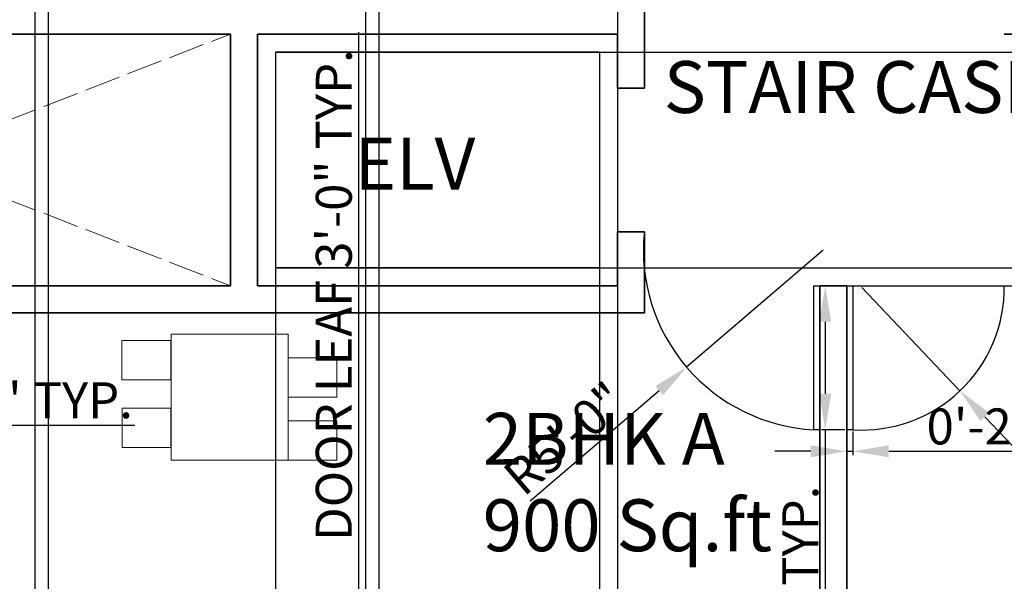
# Model space of a CAD drawing. Units: inches. Extents: x 2174 to 3353, y 1481 to 2316.
# Tile 3 of 8: x 2431 to 2759, y 1713 to 1900. Entities that reach past the tile are written whole.
import ezdxf

# ---------------------------------------------------------------- set-up
doc = ezdxf.new("R2010")
doc.units = ezdxf.units.IN
doc.linetypes.add('ACAD_ISO02W100', pattern=[15, 12, -3])
for name, color, linetype, lineweight in [('A-ANNO-DIMS', 2, 'Continuous', 18), ('A-AREA-IDEN', 7, 'Continuous', 25), ('A-DOOR', 4, 'Continuous', 25), ('A-EQPM-ELEV', 4, 'Continuous', 25), ('A-FLOR-OPEN', 8, 'ACAD_ISO02W100', 13), ('A-FURN', 8, 'Continuous', 13), ('A-WALL', 7, 'Continuous', 35)]:
    doc.layers.add(name, color=color, linetype=linetype, lineweight=lineweight)
doc.styles.get("Standard").update_dxf_attribs({"font": 'arial.ttf'})
doc.dimstyles.new('ISO-25', dxfattribs={"dimtxt": 12, "dimasz": 12, "dimexe": 1.25, "dimexo": 0.625, "dimtad": 1, "dimlunit": 3, "dimtxsty": 'Standard', "dimcen": 2.5, "dimadec": 0, "dimazin": 0, "dimtfac": 1, "dimtmove": 0, "dimatfit": 3, "dimfxl": 1, "dimarcsym": 0})

# ---------------------------------------------------------------- blocks, each defined once
blk = doc.blocks.new('DINING-SET-4')
for points in [[(0, 39.9), (16.26, 39.9), (16.26, 26.81), (0, 26.81)], [(16.43, 42.05), (55.41, 42.05), (55.41, 0), (16.43, 0)], [(55.41, 34.11), (71.67, 34.11), (71.67, 21.03), (55.41, 21.03)], [(0.02, 17.35), (16.29, 17.35), (16.29, 4.26), (0.02, 4.26)], [(55.41, 13.09), (71.67, 13.09), (71.67, 0), (55.41, 0)]]:
    blk.add_lwpolyline(points, close=True)
blk = doc.blocks.new('DOOR-LEAF-48IN')
for p, q in [((0, 0), (0, 2)), ((0, 2), (48, 2)), ((48, 0), (0, 0)), ((48, 2), (48, 0))]:
    blk.add_line(p, q)
blk = doc.blocks.new('OPENING-CROSS-18FT-7FT')
for p, q in [((0, 0), (216, 84)), ((0, 84), (216, 0))]:
    blk.add_line(p, q)
blk = doc.blocks.new('*D22')
at = {"layer": 'A-ANNO-DIMS', "color": 0, "lineweight": -2, "transparency": 16777216}
for p, q in [((2346.98, 1768.45), (2346.98, 1763.89)), ((2371.01, 1768.45), (2371.01, 1763.89)), ((2334.98, 1765.14), (2322.98, 1765.14)), ((2346.98, 1765.14), (2371.01, 1765.14)), ((2383.01, 1765.14), (2469.61, 1765.14))]:
    blk.add_line(p, q, dxfattribs=at)
at = {"layer": 'A-ANNO-DIMS', "color": 0, "transparency": 16777216}
for points in [[(2334.98, 1767.14), (2334.98, 1763.14), (2346.98, 1765.14)], [(2383.01, 1767.14), (2383.01, 1763.14), (2371.01, 1765.14)]]:
    blk.add_solid(points, dxfattribs=at)
at = {"layer": 'Defpoints', "color": 0, "transparency": 16777216}
for p in [(2346.98, 1769.07), (2371.01, 1769.07), (2371.01, 1765.14)]:
    blk.add_point(p, dxfattribs=at)
at = {"layer": 'A-ANNO-DIMS', "color": 0, "transparency": 16777216, "insert": (2432.31, 1771.89), "char_height": 12, "attachment_point": 5}
blk.add_mtext('2\'-0" TYP.', dxfattribs=at)
blk = doc.blocks.new('*D23')
at = {"layer": 'A-ANNO-DIMS', "color": 0, "lineweight": -2, "transparency": 16777216}
for p, q in [((2706.32, 1811.61), (2698.49, 1811.61)), ((2699.74, 1799.61), (2699.74, 1775.61)), ((2706.32, 1763.61), (2698.49, 1763.61)), ((2699.74, 1763.61), (2699.74, 1569.78))]:
    blk.add_line(p, q, dxfattribs=at)
at = {"layer": 'A-ANNO-DIMS', "color": 0, "transparency": 16777216}
for points in [[(2697.74, 1799.61), (2701.74, 1799.61), (2699.74, 1811.61)], [(2697.74, 1775.61), (2701.74, 1775.61), (2699.74, 1763.61)]]:
    blk.add_solid(points, dxfattribs=at)
at = {"layer": 'Defpoints', "color": 0, "transparency": 16777216}
for p in [(2706.94, 1811.61), (2699.74, 1763.61), (2706.94, 1763.61)]:
    blk.add_point(p, dxfattribs=at)
at = {"layer": 'A-ANNO-DIMS', "color": 0, "transparency": 16777216, "insert": (2692.99, 1660.7), "char_height": 12, "attachment_point": 5, "rotation": 90}
blk.add_mtext('ENTRY LEAF 4\'-0" TYP.', dxfattribs=at)
blk = doc.blocks.new('*D24')
at = {"layer": 'A-ANNO-DIMS', "color": 0, "lineweight": -2, "transparency": 16777216}
for p, q in [((2706.94, 1762.98), (2706.94, 1755.16)), ((2708.94, 1762.98), (2708.94, 1755.16)), ((2694.94, 1756.41), (2682.94, 1756.41)), ((2706.94, 1756.41), (2708.94, 1756.41)), ((2720.94, 1756.41), (2807.34, 1756.41))]:
    blk.add_line(p, q, dxfattribs=at)
at = {"layer": 'A-ANNO-DIMS', "color": 0, "transparency": 16777216}
for points in [[(2694.94, 1758.41), (2694.94, 1754.41), (2706.94, 1756.41)], [(2720.94, 1758.41), (2720.94, 1754.41), (2708.94, 1756.41)]]:
    blk.add_solid(points, dxfattribs=at)
at = {"layer": 'Defpoints', "color": 0, "transparency": 16777216}
for p in [(2706.94, 1763.61), (2708.94, 1763.61), (2708.94, 1756.41)]:
    blk.add_point(p, dxfattribs=at)
at = {"layer": 'A-ANNO-DIMS', "color": 0, "transparency": 16777216, "insert": (2770.14, 1763.16), "char_height": 12, "attachment_point": 5}
blk.add_mtext('0\'-2" TYP.', dxfattribs=at)
blk = doc.blocks.new('*D25')
at = {"layer": 'A-ANNO-DIMS', "color": 0, "lineweight": -2, "transparency": 16777216}
for p, q in [((2544.29, 1708.86), (2544.29, 1896.19)), ((2549.07, 1708.86), (2543.04, 1708.86)), ((2544.29, 1684.86), (2544.29, 1696.86)), ((2549.07, 1672.86), (2543.04, 1672.86))]:
    blk.add_line(p, q, dxfattribs=at)
at = {"layer": 'A-ANNO-DIMS', "color": 0, "transparency": 16777216}
for points in [[(2542.29, 1696.86), (2546.29, 1696.86), (2544.29, 1708.86)], [(2542.29, 1684.86), (2546.29, 1684.86), (2544.29, 1672.86)]]:
    blk.add_solid(points, dxfattribs=at)
at = {"layer": 'Defpoints', "color": 0, "transparency": 16777216}
for p in [(2544.29, 1708.86), (2549.69, 1708.86), (2549.69, 1672.86)]:
    blk.add_point(p, dxfattribs=at)
at = {"layer": 'A-ANNO-DIMS', "color": 0, "transparency": 16777216, "insert": (2537.46, 1808.52), "char_height": 12, "attachment_point": 5, "rotation": 90}
blk.add_mtext('DOOR LEAF 3\'-0" TYP.', dxfattribs=at)
blk = doc.blocks.new('*D43')
at = {"layer": 'A-ANNO-DIMS', "color": 0, "lineweight": -2, "transparency": 16777216}
for p, q in [((2707.57, 1811.61), (3156.24, 1811.61)), ((3154.99, 1565.61), (3154.99, 1799.61)), ((2707.57, 1553.61), (3156.24, 1553.61))]:
    blk.add_line(p, q, dxfattribs=at)
at = {"layer": 'A-ANNO-DIMS', "color": 0, "transparency": 16777216}
for points in [[(3152.99, 1799.61), (3156.99, 1799.61), (3154.99, 1811.61)], [(3152.99, 1565.61), (3156.99, 1565.61), (3154.99, 1553.61)]]:
    blk.add_solid(points, dxfattribs=at)
at = {"layer": 'Defpoints', "color": 0, "transparency": 16777216}
for p in [(2706.94, 1811.61), (3154.99, 1811.61), (2706.94, 1553.61)]:
    blk.add_point(p, dxfattribs=at)
at = {"layer": 'A-ANNO-DIMS', "color": 0, "transparency": 16777216, "insert": (3148.24, 1682.61), "char_height": 12, "attachment_point": 5, "rotation": 90}
blk.add_mtext('21\'-6"', dxfattribs=at)
blk = doc.blocks.new('*D49')
at = {"layer": 'A-ANNO-DIMS', "color": 0, "lineweight": -2, "transparency": 16777216}
for p, q in [((2294.44, 2143.98), (2294.44, 1510.81)), ((2436.19, 2143.98), (2436.19, 1510.81)), ((2306.44, 1512.06), (2424.19, 1512.06))]:
    blk.add_line(p, q, dxfattribs=at)
at = {"layer": 'A-ANNO-DIMS', "color": 0, "transparency": 16777216}
for points in [[(2306.44, 1514.06), (2306.44, 1510.06), (2294.44, 1512.06)], [(2424.19, 1514.06), (2424.19, 1510.06), (2436.19, 1512.06)]]:
    blk.add_solid(points, dxfattribs=at)
at = {"layer": 'Defpoints', "color": 0, "transparency": 16777216}
for p in [(2294.44, 2144.61), (2436.19, 2144.61), (2436.19, 1512.06)]:
    blk.add_point(p, dxfattribs=at)
at = {"layer": 'A-ANNO-DIMS', "color": 0, "transparency": 16777216, "insert": (2365.32, 1518.81), "char_height": 12, "attachment_point": 5}
blk.add_mtext('11\'-10"', dxfattribs=at)
blk = doc.blocks.new('*D50')
at = {"layer": 'A-ANNO-DIMS', "color": 0, "lineweight": -2, "transparency": 16777216}
for p, q in [((2440.69, 2143.98), (2440.69, 1510.81)), ((2546.44, 2143.98), (2546.44, 1510.81)), ((2452.69, 1512.06), (2534.44, 1512.06))]:
    blk.add_line(p, q, dxfattribs=at)
at = {"layer": 'A-ANNO-DIMS', "color": 0, "transparency": 16777216}
for points in [[(2452.69, 1514.06), (2452.69, 1510.06), (2440.69, 1512.06)], [(2534.44, 1514.06), (2534.44, 1510.06), (2546.44, 1512.06)]]:
    blk.add_solid(points, dxfattribs=at)
at = {"layer": 'Defpoints', "color": 0, "transparency": 16777216}
for p in [(2440.69, 2144.61), (2546.44, 2144.61), (2546.44, 1512.06)]:
    blk.add_point(p, dxfattribs=at)
at = {"layer": 'A-ANNO-DIMS', "color": 0, "transparency": 16777216, "insert": (2493.57, 1518.81), "char_height": 12, "attachment_point": 5}
blk.add_mtext('8\'-10"', dxfattribs=at)
blk = doc.blocks.new('*D51')
at = {"layer": 'A-ANNO-DIMS', "color": 0, "lineweight": -2, "transparency": 16777216}
for p, q in [((2550.94, 2143.98), (2550.94, 1510.81)), ((2630.44, 2143.98), (2630.44, 1510.81)), ((2562.94, 1512.06), (2618.44, 1512.06))]:
    blk.add_line(p, q, dxfattribs=at)
at = {"layer": 'A-ANNO-DIMS', "color": 0, "transparency": 16777216}
for points in [[(2562.94, 1514.06), (2562.94, 1510.06), (2550.94, 1512.06)], [(2618.44, 1514.06), (2618.44, 1510.06), (2630.44, 1512.06)]]:
    blk.add_solid(points, dxfattribs=at)
at = {"layer": 'Defpoints', "color": 0, "transparency": 16777216}
for p in [(2550.94, 2144.61), (2630.44, 2144.61), (2630.44, 1512.06)]:
    blk.add_point(p, dxfattribs=at)
at = {"layer": 'A-ANNO-DIMS', "color": 0, "transparency": 16777216, "insert": (2590.69, 1518.89), "char_height": 12, "attachment_point": 5}
blk.add_mtext('6\'-7 1/2"', dxfattribs=at)
blk = doc.blocks.new('*D60')
at = {"layer": 'A-ANNO-DIMS', "color": 0, "lineweight": -2, "transparency": 16777216}
for p, q in [((2516.44, 1888.98), (2516.44, 1510.81)), ((2624.44, 1888.98), (2624.44, 1510.81)), ((2528.44, 1512.06), (2612.44, 1512.06))]:
    blk.add_line(p, q, dxfattribs=at)
at = {"layer": 'A-ANNO-DIMS', "color": 0, "transparency": 16777216}
for points in [[(2528.44, 1514.06), (2528.44, 1510.06), (2516.44, 1512.06)], [(2612.44, 1514.06), (2612.44, 1510.06), (2624.44, 1512.06)]]:
    blk.add_solid(points, dxfattribs=at)
at = {"layer": 'Defpoints', "color": 0, "transparency": 16777216}
for p in [(2516.44, 1889.61), (2624.44, 1889.61), (2624.44, 1512.06)]:
    blk.add_point(p, dxfattribs=at)
at = {"layer": 'A-ANNO-DIMS', "color": 0, "transparency": 16777216, "insert": (2570.44, 1518.81), "char_height": 12, "attachment_point": 5}
blk.add_mtext('9\'-0"', dxfattribs=at)
blk = doc.blocks.new('*D61')
at = {"layer": 'A-ANNO-DIMS', "color": 0, "lineweight": -2, "transparency": 16777216}
for p, q in [((2517.07, 1889.61), (3156.24, 1889.61)), ((3154.99, 1829.61), (3154.99, 1877.61)), ((2517.07, 1817.61), (3156.24, 1817.61))]:
    blk.add_line(p, q, dxfattribs=at)
at = {"layer": 'A-ANNO-DIMS', "color": 0, "transparency": 16777216}
for points in [[(3152.99, 1877.61), (3156.99, 1877.61), (3154.99, 1889.61)], [(3152.99, 1829.61), (3156.99, 1829.61), (3154.99, 1817.61)]]:
    blk.add_solid(points, dxfattribs=at)
at = {"layer": 'Defpoints', "color": 0, "transparency": 16777216}
for p in [(2516.44, 1889.61), (3154.99, 1889.61), (2516.44, 1817.61)]:
    blk.add_point(p, dxfattribs=at)
at = {"layer": 'A-ANNO-DIMS', "color": 0, "transparency": 16777216, "insert": (3148.24, 1853.61), "char_height": 12, "attachment_point": 5, "rotation": 90}
blk.add_mtext('6\'-0"', dxfattribs=at)
blk = doc.blocks.new('*D76')
at = {"layer": 'A-ANNO-DIMS', "color": 0, "lineweight": -2, "transparency": 16777216}
for p, q in [((2699.06, 1823.46), (2653.53, 1784.48)), ((2601.39, 1739.85), (2644.42, 1776.68))]:
    blk.add_line(p, q, dxfattribs=at)
at = {"layer": 'A-ANNO-DIMS', "color": 0, "transparency": 16777216}
blk.add_solid([(2643.12, 1778.2), (2645.72, 1775.16), (2653.53, 1784.48)], dxfattribs=at)
at = {"layer": 'Defpoints', "color": 0, "transparency": 16777216}
for p in [(2699.06, 1823.46), (2653.53, 1784.48)]:
    blk.add_point(p, dxfattribs=at)
at = {"layer": 'A-ANNO-DIMS', "color": 0, "transparency": 16777216, "insert": (2613.96, 1759.49), "char_height": 12, "attachment_point": 5, "rotation": 40.566}
blk.add_mtext('R5\'-0"', dxfattribs=at)
blk = doc.blocks.new('*D77')
at = {"layer": 'A-ANNO-DIMS', "color": 0, "lineweight": -2, "transparency": 16777216}
for p, q in [((2711.9, 1811.07), (2744.66, 1776.6)), ((2817.63, 1699.83), (2752.92, 1767.9))]:
    blk.add_line(p, q, dxfattribs=at)
at = {"layer": 'A-ANNO-DIMS', "color": 0, "transparency": 16777216}
blk.add_solid([(2754.37, 1769.28), (2751.47, 1766.52), (2744.66, 1776.6)], dxfattribs=at)
at = {"layer": 'Defpoints', "color": 0, "transparency": 16777216}
for p in [(2711.9, 1811.07), (2744.66, 1776.6)]:
    blk.add_point(p, dxfattribs=at)
at = {"layer": 'A-ANNO-DIMS', "color": 0, "transparency": 16777216, "insert": (2794.36, 1734.22), "char_height": 12, "attachment_point": 5, "rotation": 313.546}
blk.add_mtext('R3\'-11 1/2"', dxfattribs=at)

msp = doc.modelspace()

# ---------------------------------------------------------------- linework, layer by layer
at = {"layer": 'A-DOOR'}
for centre, radius, start, end in [((2699.062, 1823.46), 59.934, 174.11259, 267.01847), ((2711.898, 1811.065), 47.549, 266.43858, 0.65363)]:
    msp.add_arc(centre, radius, start, end, dxfattribs=at)
at = {"layer": 'A-EQPM-ELEV'}
for p, q in [((2516.444, 1889.608), (2516.444, 1817.608)), ((2624.444, 1889.608), (2516.444, 1889.608)), ((2624.444, 1889.608), (2624.444, 1817.608)), ((2624.444, 1817.608), (2516.444, 1817.608))]:
    msp.add_line(p, q, dxfattribs=at)
at = {"layer": 'A-WALL'}
for p, q in [((2639.444, 1904.608), (2639.444, 1895.608)), ((2501.444, 1895.608), (2285.444, 1895.608)), ((2501.444, 1895.608), (2501.444, 1811.608)), ((2630.444, 1895.608), (2510.444, 1895.608)), ((2510.444, 1895.608), (2510.444, 1811.608)), ((2630.444, 1895.608), (2630.444, 1877.608)), ((2639.444, 1895.608), (2639.444, 1877.608)), ((2759.444, 1895.608), (2795.444, 1895.608)), ((2630.444, 1877.608), (2639.444, 1877.608)), ((2630.444, 1829.608), (2639.444, 1829.608)), ((2630.444, 1829.608), (2630.444, 1811.608)), ((2639.444, 1829.608), (2639.444, 1802.608)), ((2501.444, 1811.608), (2285.444, 1811.608)), ((2630.444, 1811.608), (2510.444, 1811.608)), ((2697.944, 1811.608), (2706.944, 1811.608)), ((2697.944, 1562.608), (2697.944, 1811.608)), ((2706.944, 1553.608), (2706.944, 1811.608)), ((2639.444, 1802.608), (2392.694, 1802.608))]:
    msp.add_line(p, q, dxfattribs=at)

# ---------------------------------------------------------------- block references
at = {"layer": 'A-DOOR'}
for p, rotation in [((2697.944, 1763.608), 90.0000000000016), ((2706.944, 1811.608), 270.0000000000017)]:
    msp.add_blockref('DOOR-LEAF-48IN', p, dxfattribs=dict(at, rotation=rotation))
at = {"layer": 'A-FLOR-OPEN'}
msp.add_blockref('OPENING-CROSS-18FT-7FT', (2285.444, 1811.608), dxfattribs=at)
at = {"layer": 'A-FURN'}
msp.add_blockref('DINING-SET-4', (2465.293, 1753.459), dxfattribs=at)

# ---------------------------------------------------------------- texts
at = {"layer": 'A-AREA-IDEN', "char_height": 17.3039, "attachment_point": 1}
for s, insert in [('STAIR CASE', (2645.911, 1886.581)), ('ELV', (2542.784, 1861.026)), ('2BHK A\\P900 Sq.ft', (2585.567, 1769.24))]:
    msp.add_mtext_dynamic_manual_height_columns(s, width=375.7284, gutter_width=86.519, heights=[0], dxfattribs=dict(at, insert=insert))

# ---------------------------------------------------------------- dimensions: what is measured, and where the dimension line sits
at = {"layer": 'A-ANNO-DIMS'}
for base, p1, p2, picture, middle in [((2436.194421, 1512.057615), (2294.444421, 2144.607615), (2436.194421, 2144.607615), '*D49', (2365.319421, 1518.809490853)), ((2546.444421, 1512.057615), (2440.694421, 2144.607615), (2546.444421, 2144.607615), '*D50', (2493.569421, 1518.809490853)), ((2630.444, 1512.058), (2550.944, 2144.608), (2630.444, 2144.608), '*D51', (2590.694, 1518.887)), ((2624.444, 1512.058), (2516.444, 1889.608), (2624.444, 1889.608), '*D60', (2570.444, 1518.809))]:
    dim = msp.add_linear_dim(base=base, p1=p1, p2=p2, dimstyle='ISO-25', override={"dimdec": 1, "dimlfac": 1, "dimrnd": 0, "dimzin": 1, "dimdsep": 46, "dimlunit": 4, "dimfrac": 2}, dxfattribs=at)
    dim.commit()
    dim.dimension.update_dxf_attribs({"geometry": picture, "text_midpoint": middle})
for base, p1, p2, angle, text, picture, middle in [((2544.294, 1708.858), (2549.694, 1672.858), (2549.694, 1708.858), 90, 'DOOR LEAF <> TYP.', '*D25', (2537.457, 1808.524)), ((2699.744, 1763.608), (2706.944, 1811.608), (2706.944, 1763.608), 270, 'ENTRY LEAF <> TYP.', '*D23', (2692.993, 1660.696))]:
    dim = msp.add_linear_dim(base=base, p1=p1, p2=p2, angle=angle, text=text, dimstyle='ISO-25', override={"dimdec": 1, "dimlfac": 1, "dimrnd": 0, "dimzin": 1, "dimdsep": 46, "dimlunit": 4, "dimfrac": 2}, dxfattribs=at)
    dim.commit()
    dim.dimension.update_dxf_attribs({"geometry": picture, "text_midpoint": middle})
for base, p1, p2, picture, middle in [((3154.994, 1889.608), (2516.444, 1817.608), (2516.444, 1889.608), '*D61', (3148.243, 1853.608)), ((3154.994, 1811.608), (2706.944, 1553.608), (2706.944, 1811.608), '*D43', (3148.243, 1682.608))]:
    dim = msp.add_linear_dim(base=base, p1=p1, p2=p2, angle=90, dimstyle='ISO-25', override={"dimdec": 1, "dimlfac": 1, "dimrnd": 0, "dimzin": 1, "dimdsep": 46, "dimlunit": 4, "dimfrac": 2}, dxfattribs=at)
    dim.commit()
    dim.dimension.update_dxf_attribs({"geometry": picture, "text_midpoint": middle})
for center, mpoint, picture, middle in [((2699.062, 1823.46), (2653.533, 1784.484), '*D76', (2613.957, 1759.492)), ((2711.898, 1811.065), (2744.657, 1776.6), '*D77', (2794.363, 1734.225))]:
    dim = msp.add_radius_dim(center=center, mpoint=mpoint, dimstyle='ISO-25', override={"dimdec": 1, "dimlfac": 1, "dimrnd": 0, "dimzin": 1, "dimdsep": 46, "dimlunit": 4, "dimfrac": 2}, dxfattribs=at)
    dim.commit()
    dim.dimension.update_dxf_attribs({"geometry": picture, "text_midpoint": middle})
for base, p1, p2, picture, middle in [((2371.005, 1765.138), (2346.979, 1769.075), (2371.005, 1769.075), '*D22', (2432.305, 1771.89)), ((2708.944, 1756.408), (2706.944, 1763.608), (2708.944, 1763.608), '*D24', (2770.142, 1763.159))]:
    dim = msp.add_linear_dim(base=base, p1=p1, p2=p2, text='<> TYP.', dimstyle='ISO-25', override={"dimdec": 1, "dimlfac": 1, "dimrnd": 0, "dimzin": 1, "dimdsep": 46, "dimlunit": 4, "dimfrac": 2}, dxfattribs=at)
    dim.commit()
    dim.dimension.update_dxf_attribs({"geometry": picture, "text_midpoint": middle})

doc.saveas('drawing.dxf')
